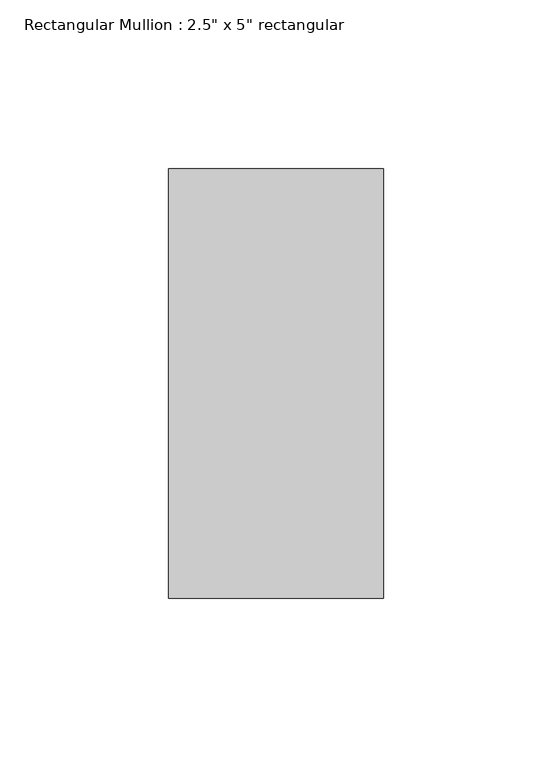
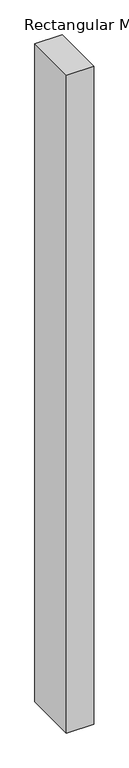
"""IFC4 building model written with IfcOpenShell, lengths in millimetres: member geometry."""

from ifc_helpers import new_model, si_unit, frame, origin, place, context, project, spatial, polyline, outline, extrude, source, transform, mapped, element, save


def member_8a463cd0(model_context):
    return source(origin(), model_context, "Body", "SweptSolid", [
        extrude(outline(polyline([(0.0, 63.5), (0.0, -63.5), (-63.5, -63.5), (-63.5, 63.5), (0.0, 63.5)])), frame((0.0, 0.0, -1620.8138027), z_axis=(0.0, 0.0, 1.0), x_axis=(1.0, 0.0, 0.0)), (0.0, 0.0, 1.0), 1620.8138027),
    ])


if __name__ == "__main__":
    model = new_model("IFC4")
    model_context = context("Model", 3, world=origin())
    ifc_project = project(units=[si_unit("LENGTHUNIT", "METRE", prefix="MILLI")], contexts=[model_context])
    site = spatial("IfcSite", under=ifc_project)
    building = spatial("IfcBuilding", under=site)
    placement = place(None, origin())
    member_shape = member_8a463cd0(model_context)
    element("IfcMember", 1, ObjectType="Rectangular Mullion : 2.5\" x 5\" rectangular", at=placement, inside=building, context=model_context, shape_type="MappedRepresentation", body=[
        mapped(member_shape, transform((0.0, 0.0, 0.0), x_axis=(1.0, 0.0, 0.0), y_axis=(0.0, 1.0, 0.0), z_axis=(0.0, 0.0, 1.0))),
    ])
    save(model, "model.ifc")

# Revit data of these elements
# Type "Rectangular Mullion : 2.5\" x 5\" rectangular"
#   built-in parameter 1007304 = 0.416667 (stored number, unit not read)
#   built-in parameter 1007301 = 0.104167 (stored number, unit not read)
#   built-in parameter 1007300 = 0.104167 (stored number, unit not read)
# Element 1 (IfcMember, "Rectangular Mullion : 2.5\" x 5\" rectangular")
#   Materials on its faces: "Aluminum"
# Materials
#   "Aluminum": class "Metal", colour RGB 247 247 247, transparency 0, Description = "Aluminum 6061", Cost = 0
